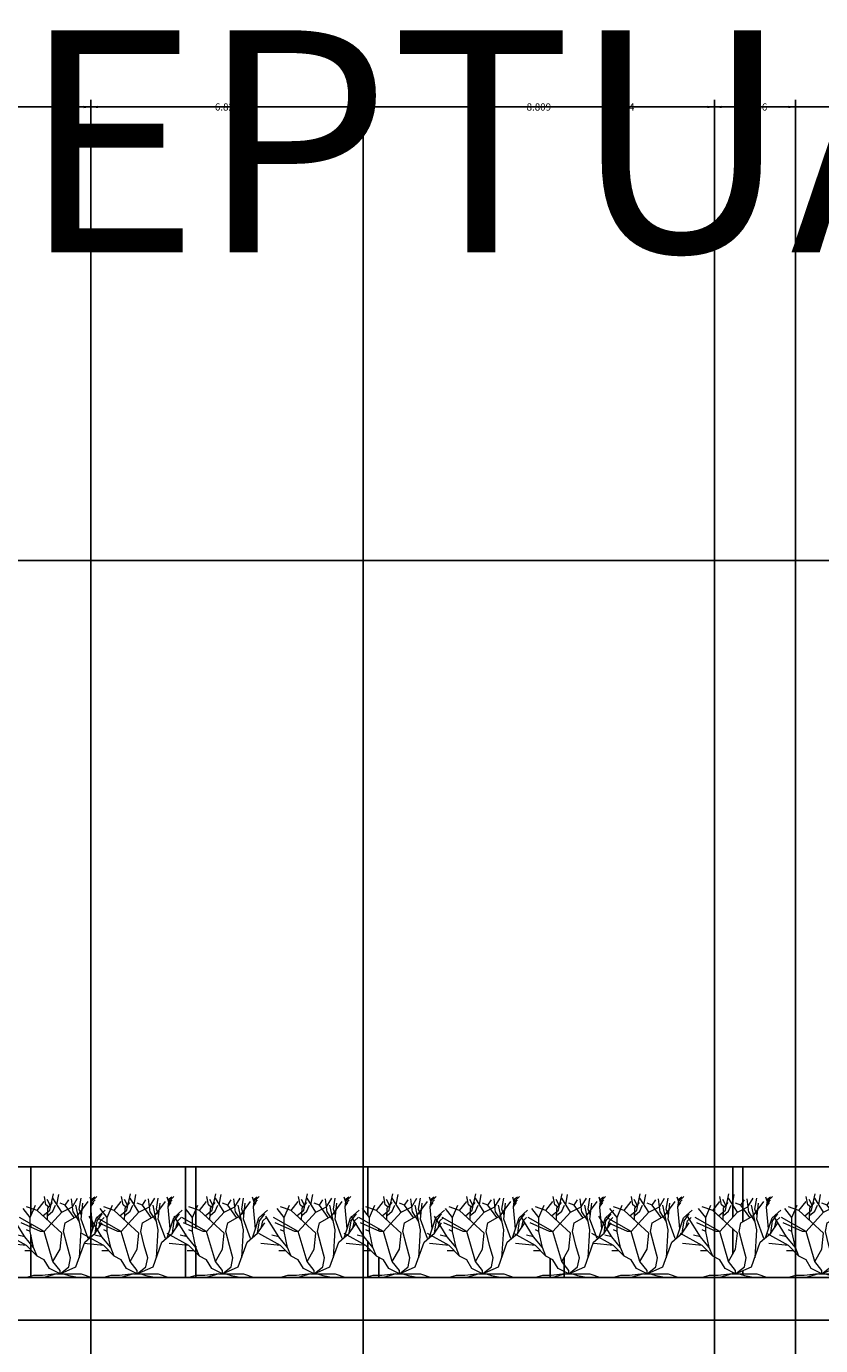
# Model space of a CAD drawing. Units: inches. Extents: x -117 to 121, y -77 to 40.
# Tile 16 of 45: x -65 to -45, y 7 to 40. Entities that reach past the tile are written whole.
import ezdxf

# ---------------------------------------------------------------- set-up
doc = ezdxf.new("R2010")
doc.units = ezdxf.units.IN
doc.header["$MEASUREMENT"] = 0
for name, color, linetype, lineweight in [('A-ANNO-DIMS', 2, 'Continuous', 18), ('A-ANNO-TEXT', 7, 'Continuous', 25), ('A-ELEV', 7, 'Continuous', 25), ('L-PLNT', 3, 'Continuous', 13)]:
    doc.layers.add(name, color=color, linetype=linetype, lineweight=lineweight)
doc.styles.get("Standard").update_dxf_attribs({"font": 'arial.ttf'})
doc.dimstyles.get("Standard").update_dxf_attribs({"dimtxt": 0.18, "dimasz": 0.18, "dimexe": 0.18, "dimexo": 0.0625, "dimgap": 0.09, "dimtad": 0, "dimtih": 1, "dimtoh": 1, "dimdec": 4, "dimzin": 0, "dimdsep": 46, "dimtxsty": 'Standard', "dimcen": 0.09, "dimadec": 0, "dimazin": 0, "dimtfac": 1, "dimtdec": 4, "dimtofl": 0, "dimtmove": 0, "dimatfit": 3, "dimfxl": 1, "dimtolj": 1, "dimtzin": 0, "dimarcsym": 0})

# ---------------------------------------------------------------- blocks, each defined once
blk = doc.blocks.new('*U3')
for p, q in [((-12.471, 19.775), (-12.898, 22.044)), ((-11.433, 18.289), (-10.457, 22.749)), ((-8.16, 17.76), (-10.56, 21.6)), ((-9.48, 19.775), (-8.992, 22.592)), ((-5.28, 19.2), (-3.84, 21.6)), ((-3.377, 18.602), (-2.888, 21.575)), ((-0.508, 21.888), (-0.081, 20.558)), ((0.041, 20.714), (1.384, 22.044)), ((0.102, 21.34), (0.835, 21.888)), ((-16.8, 16.32), (-18.72, 18.72)), ((-14.88, 18.24), (-17.76, 19.2)), ((-16.8, 16.32), (-15.36, 19.68)), ((-14.88, 18.24), (-12.96, 20.64)), ((-8.16, 12), (-14.88, 18.24)), ((-13.325, 16.724), (-11.433, 18.289)), ((-11.677, 19.071), (-12.471, 19.775)), ((-11.28, 19.619), (-12.104, 21.184)), ((-12.043, 15.628), (-11.921, 18.836)), ((-11.982, 16.802), (-10.579, 18.054)), ((-11.921, 18.836), (-10.64, 20.401)), ((-10.579, 18.054), (-9.846, 19.697)), ((-7.2, 19.68), (-8.64, 20.16)), ((-8.16, 17.76), (-5.28, 19.2)), ((-7.2, 19.68), (-6.24, 21.12)), ((-4.8, 16.32), (-7.2, 19.68)), ((-5.086, 17.741), (-5.513, 21.34)), ((-2.88, 12.96), (-4.32, 19.68)), ((-3.84, 16.8), (-0.96, 20.64)), ((-2.766, 16.802), (-3.377, 18.602)), ((-2.88, 15.84), (-2.4, 20.16)), ((-0.203, 19.149), (0.102, 21.34)), ((0.346, 13.203), (-0.203, 19.149)), ((-0.142, 19.384), (0.59, 20.401)), ((-0.02, 20.01), (0.896, 21.105)), ((1.323, 16.254), (3.642, 18.289)), ((-18.24, 11.04), (-21.755, 16.655)), ((-12.96, 12.48), (-19.68, 16.32)), ((-13.92, 12.48), (-19.2, 14.88)), ((-16.8, 12.48), (-16.8, 16.32)), ((-12.96, 12.48), (-8.16, 17.76)), ((-7.68, 12.48), (-7.2, 14.88)), ((-7.2, 14.88), (-3.84, 16.8)), ((-3.377, 15.315), (-5.086, 17.819)), ((-0.96, 10.56), (-2.88, 15.84)), ((0.346, 13.203), (1.323, 16.254)), ((0.96, 12), (1.44, 15.36)), ((0.96, 12), (2.88, 14.88)), ((1.44, 15.36), (2.88, 17.28)), ((1.92, 13.44), (2.4, 15.36)), ((2.4, 15.36), (3.36, 16.32)), ((-17.76, 8.64), (-23.663, 11.961)), ((-18.24, 11.04), (-20.16, 11.52)), ((-15.84, 8.16), (-18.24, 11.04)), ((-16.8, 12.48), (-17.76, 12.96)), ((-15.84, 8.16), (-16.8, 12.48)), ((-12.96, 12.48), (-13.92, 12.48)), ((-10.56, 4.32), (-12.96, 12.48)), ((-8.64, 7.68), (-8.16, 12)), ((-6.72, 8.64), (-7.68, 12.48)), ((-3.36, 5.28), (-2.88, 12.96)), ((-1.92, 9.6), (0.96, 12)), ((-0.48, 10.8), (0.346, 13.203)), ((-17.76, 8.64), (-23.128, 9.222)), ((-16.32, 7.2), (-18.24, 7.2)), ((-14.88, 5.76), (-17.76, 8.64)), ((-14.88, 5.76), (-15.84, 8.16)), ((-10.56, 4.32), (-8.64, 7.68)), ((-5.76, 5.28), (-6.72, 8.64)), ((-4.32, 2.88), (-1.92, 9.6)), ((-12.96, 4.8), (-14.88, 5.76)), ((-11.52, 2.4), (-12.96, 4.8)), ((-8.64, 1.92), (-10.56, 4.32)), ((-6.24, 2.88), (-5.76, 5.28)), ((-15.84, 0.48), (-17.76, 0)), ((-13.44, 0.48), (-15.84, 0.48)), ((-9.6, 0.96), (-13.44, 0.48)), ((-9.6, 0.96), (-12.96, 0)), ((-8.64, 0.96), (-11.52, 2.4)), ((-9.6, 0.96), (-7.68, 0.96)), ((-8.64, 0.96), (-4.32, 2.88)), ((-8.64, 0.96), (-6.24, 2.88)), ((-8.64, 0.96), (-8.64, 1.92)), ((-8.64, 0.96), (-2.88, 0.96)), ((-7.68, 0.96), (-6.24, 0.48)), ((-6.24, 0.48), (-3.36, 0)), ((-2.88, 0.96), (0, 0))]:
    blk.add_line(p, q)
blk = doc.blocks.new('*D9')
at = {"layer": 'A-ANNO-DIMS', "color": 0, "lineweight": -2, "transparency": 16777216}
for p, q in [((-75.804, 8.087), (-75.804, 38.61)), ((-75.624, 38.43), (-50.227, 38.43)), ((-24.044, 38.43), (-49.44, 38.43)), ((-23.864, 8.087), (-23.864, 38.61))]:
    blk.add_line(p, q, dxfattribs=at)
at = {"layer": 'A-ANNO-DIMS', "color": 0, "transparency": 16777216}
for points in [[(-75.624, 38.46), (-75.624, 38.4), (-75.804, 38.43)], [(-24.044, 38.46), (-24.044, 38.4), (-23.864, 38.43)]]:
    blk.add_solid(points, dxfattribs=at)
at = {"layer": 'Defpoints', "color": 0, "transparency": 16777216}
for p in [(-23.864, 38.43), (-75.804, 8.025), (-23.864, 8.025)]:
    blk.add_point(p, dxfattribs=at)
at = {"layer": 'A-ANNO-DIMS', "color": 0, "transparency": 16777216, "insert": (-49.834, 38.43), "char_height": 0.18, "attachment_point": 5}
blk.add_mtext('\\A1;51.94', dxfattribs=at)
blk = doc.blocks.new('*D13')
at = {"layer": 'A-ANNO-DIMS', "color": 0, "lineweight": -2, "transparency": 16777216}
for p, q in [((-2.663, 27.063), (-117.024, 27.063)), ((-116.844, 26.883), (-116.844, -16.974)), ((-116.844, -61.196), (-116.844, -17.338)), ((-106.096, -61.376), (-117.024, -61.376))]:
    blk.add_line(p, q, dxfattribs=at)
at = {"layer": 'A-ANNO-DIMS', "color": 0, "transparency": 16777216}
for points in [[(-116.874, 26.883), (-116.814, 26.883), (-116.844, 27.063)], [(-116.874, -61.196), (-116.814, -61.196), (-116.844, -61.376)]]:
    blk.add_solid(points, dxfattribs=at)
at = {"layer": 'Defpoints', "color": 0, "transparency": 16777216}
for p in [(-2.6, 27.063), (-116.844, -61.376), (-106.034, -61.376)]:
    blk.add_point(p, dxfattribs=at)
at = {"layer": 'A-ANNO-DIMS', "color": 0, "transparency": 16777216, "insert": (-116.844, -17.156), "char_height": 0.18, "attachment_point": 5}
blk.add_mtext('\\A1;88.44', dxfattribs=at)
blk = doc.blocks.new('*D40')
at = {"layer": 'A-ANNO-DIMS', "color": 0, "lineweight": -2, "transparency": 16777216}
for p, q in [((-86.023, -13.677), (-86.023, 38.61)), ((-85.843, 38.43), (-75.056, 38.43)), ((-63.339, 38.43), (-74.126, 38.43)), ((-63.159, -13.677), (-63.159, 38.61))]:
    blk.add_line(p, q, dxfattribs=at)
at = {"layer": 'A-ANNO-DIMS', "color": 0, "transparency": 16777216}
for points in [[(-85.843, 38.46), (-85.843, 38.4), (-86.023, 38.43)], [(-63.339, 38.46), (-63.339, 38.4), (-63.159, 38.43)]]:
    blk.add_solid(points, dxfattribs=at)
at = {"layer": 'Defpoints', "color": 0, "transparency": 16777216}
for p in [(-63.159, 38.43), (-86.023, -13.74), (-63.159, -13.74)]:
    blk.add_point(p, dxfattribs=at)
at = {"layer": 'A-ANNO-DIMS', "color": 0, "transparency": 16777216, "insert": (-74.591, 38.43), "char_height": 0.18, "attachment_point": 5}
blk.add_mtext('\\A1;22.864', dxfattribs=at)
blk = doc.blocks.new('*D41')
at = {"layer": 'A-ANNO-DIMS', "color": 0, "lineweight": -2, "transparency": 16777216}
for p, q in [((-63.159, -13.677), (-63.159, 38.61)), ((-62.979, 38.43), (-60.139, 38.43)), ((-56.51, 38.43), (-59.35, 38.43)), ((-56.33, -13.677), (-56.33, 38.61))]:
    blk.add_line(p, q, dxfattribs=at)
at = {"layer": 'A-ANNO-DIMS', "color": 0, "transparency": 16777216}
for points in [[(-62.979, 38.46), (-62.979, 38.4), (-63.159, 38.43)], [(-56.51, 38.46), (-56.51, 38.4), (-56.33, 38.43)]]:
    blk.add_solid(points, dxfattribs=at)
at = {"layer": 'Defpoints', "color": 0, "transparency": 16777216}
for p in [(-56.33, 38.43), (-63.159, -13.74), (-56.33, -13.74)]:
    blk.add_point(p, dxfattribs=at)
at = {"layer": 'A-ANNO-DIMS', "color": 0, "transparency": 16777216, "insert": (-59.744, 38.43), "char_height": 0.18, "attachment_point": 5}
blk.add_mtext('\\A1;6.829', dxfattribs=at)
blk = doc.blocks.new('*D42')
at = {"layer": 'A-ANNO-DIMS', "color": 0, "lineweight": -2, "transparency": 16777216}
for p, q in [((-56.33, -13.677), (-56.33, 38.61)), ((-56.15, 38.43), (-52.319, 38.43)), ((-47.701, 38.43), (-51.531, 38.43)), ((-47.521, -13.677), (-47.521, 38.61))]:
    blk.add_line(p, q, dxfattribs=at)
at = {"layer": 'A-ANNO-DIMS', "color": 0, "transparency": 16777216}
for points in [[(-56.15, 38.46), (-56.15, 38.4), (-56.33, 38.43)], [(-47.701, 38.46), (-47.701, 38.4), (-47.521, 38.43)]]:
    blk.add_solid(points, dxfattribs=at)
at = {"layer": 'Defpoints', "color": 0, "transparency": 16777216}
for p in [(-47.521, 38.43), (-56.33, -13.74), (-47.521, -13.74)]:
    blk.add_point(p, dxfattribs=at)
at = {"layer": 'A-ANNO-DIMS', "color": 0, "transparency": 16777216, "insert": (-51.925, 38.43), "char_height": 0.18, "attachment_point": 5}
blk.add_mtext('\\A1;8.809', dxfattribs=at)
blk = doc.blocks.new('*D43')
at = {"layer": 'A-ANNO-DIMS', "color": 0, "lineweight": -2, "transparency": 16777216}
for p, q in [((-47.521, -13.677), (-47.521, 38.61)), ((-47.341, 38.43), (-46.898, 38.43)), ((-45.665, 38.43), (-46.108, 38.43)), ((-45.485, -12.071), (-45.485, 38.61))]:
    blk.add_line(p, q, dxfattribs=at)
at = {"layer": 'A-ANNO-DIMS', "color": 0, "transparency": 16777216}
for points in [[(-47.341, 38.46), (-47.341, 38.4), (-47.521, 38.43)], [(-45.665, 38.46), (-45.665, 38.4), (-45.485, 38.43)]]:
    blk.add_solid(points, dxfattribs=at)
at = {"layer": 'Defpoints', "color": 0, "transparency": 16777216}
for p in [(-45.485, 38.43), (-45.485, -12.133), (-47.521, -13.74)]:
    blk.add_point(p, dxfattribs=at)
at = {"layer": 'A-ANNO-DIMS', "color": 0, "transparency": 16777216, "insert": (-46.503, 38.43), "char_height": 0.18, "attachment_point": 5}
blk.add_mtext('\\A1;2.036', dxfattribs=at)

msp = doc.modelspace()

# ---------------------------------------------------------------- linework, layer by layer
at = {"layer": 'A-ELEV'}
for p, q in [((-75.8037, 11.8711), (-23.8637, 11.8711)), ((-64.6661, 10.6481), (-64.6661, 11.8711)), ((-60.7913, 10.4484), (-60.7913, 11.8711)), ((-60.5325, 10.3308), (-60.5325, 11.8711)), ((-56.2143, 10.6491), (-56.2143, 11.8711)), ((-47.0603, 10.6066), (-47.0603, 11.8711)), ((-46.811, 10.4942), (-46.811, 11.8711)), ((-64.6661, 10.3582), (-64.6661, 10.4373)), ((-55.9395, 10.2602), (-55.9395, 10.3142)), ((-47.0603, 9.6811), (-47.0603, 10.3095)), ((-64.6661, 9.0994), (-64.6661, 10.1552)), ((-60.7913, 10.1257), (-60.7913, 10.1869)), ((-60.7913, 9.0994), (-60.7913, 9.9438)), ((-56.2143, 9.0994), (-56.2143, 10.0019)), ((-60.5325, 9.0994), (-60.5325, 9.8834)), ((-55.9395, 9.0994), (-55.9395, 9.5986)), ((-51.2891, 9.0994), (-51.2891, 9.6012)), ((-51.6373, 9.0994), (-51.6373, 9.5733)), ((-46.811, 9.1562), (-46.811, 9.2657)), ((-23.8637, 9.0994), (-75.8037, 9.0994)), ((-47.0603, 9.1863), (-47.0603, 9.2217)), ((-23.8637, 8.0246), (-75.8037, 8.0246))]:
    msp.add_line(p, q, dxfattribs=at)

# ---------------------------------------------------------------- block references
at = {"layer": 'L-PLNT', "xscale": 0.0920717077623056, "yscale": 0.0920717077623056, "zscale": 0.0920717077623056}
for p in [(-63.1397, 9.0979), (-61.2049, 9.0979), (-59.0664, 9.0979), (-56.7671, 9.0979), (-54.6286, 9.0979), (-52.5411, 9.0979), (-50.3772, 9.0979), (-48.4169, 9.0979), (-46.1941, 9.0979), (-44.0301, 9.0979)]:
    msp.add_blockref('*U3', p, dxfattribs=at)

# ---------------------------------------------------------------- texts
at = {"layer": 'A-ANNO-TEXT'}
msp.add_text('CONCEPTUAL    GOOD   VIBE   CAFE   DESIGN', height=5.56486, dxfattribs=at).set_placement((-85.726, 34.7863))

# ---------------------------------------------------------------- dimensions: what is measured, and where the dimension line sits
at = {"layer": 'A-ANNO-DIMS'}
for base, p1, p2, override, picture, middle in [((-63.1589, 38.4297), (-86.0225, -13.74), (-63.1589, -13.74), {"dimdec": 3, "dimlfac": 1, "dimrnd": 0, "dimzin": 0, "dimdsep": 46, "dimlunit": 2}, '*D40', (-74.5907, 38.4297)), ((-23.8637, 38.4297), (-75.8037, 8.0246), (-23.8637, 8.0246), {"dimdec": 2, "dimlfac": 1, "dimrnd": 0, "dimzin": 0, "dimdsep": 46, "dimlunit": 2}, '*D9', (-49.8337, 38.4297)), ((-56.3295, 38.4297), (-63.1589, -13.74), (-56.3295, -13.74), {"dimdec": 3, "dimlfac": 1, "dimrnd": 0, "dimzin": 0, "dimdsep": 46, "dimlunit": 2}, '*D41', (-59.7442, 38.4297)), ((-47.5206, 38.4297), (-56.3295, -13.74), (-47.5206, -13.74), {"dimdec": 3, "dimlfac": 1, "dimrnd": 0, "dimzin": 0, "dimdsep": 46, "dimlunit": 2}, '*D42', (-51.9251, 38.4297)), ((-45.4848, 38.4297), (-47.5206, -13.74), (-45.4848, -12.1334), {"dimdec": 3, "dimlfac": 1, "dimrnd": 0, "dimzin": 0, "dimdsep": 46, "dimlunit": 2}, '*D43', (-46.5027, 38.4297))]:
    dim = msp.add_linear_dim(base=base, p1=p1, p2=p2, dimstyle='Standard', override=override, dxfattribs=at)
    dim.commit()
    dim.dimension.update_dxf_attribs({"geometry": picture, "text_midpoint": middle})
dim = msp.add_linear_dim(base=(-116.8438, -61.3756), p1=(-2.6001, 27.0634), p2=(-106.0338, -61.3756), angle=90, dimstyle='Standard', override={"dimdec": 2, "dimlfac": 1, "dimrnd": 0, "dimzin": 0, "dimdsep": 46, "dimlunit": 2}, dxfattribs=at)
dim.commit()
dim.dimension.update_dxf_attribs({"geometry": '*D13', "text_midpoint": (-116.8438, -17.1561)})

doc.saveas('drawing.dxf')
